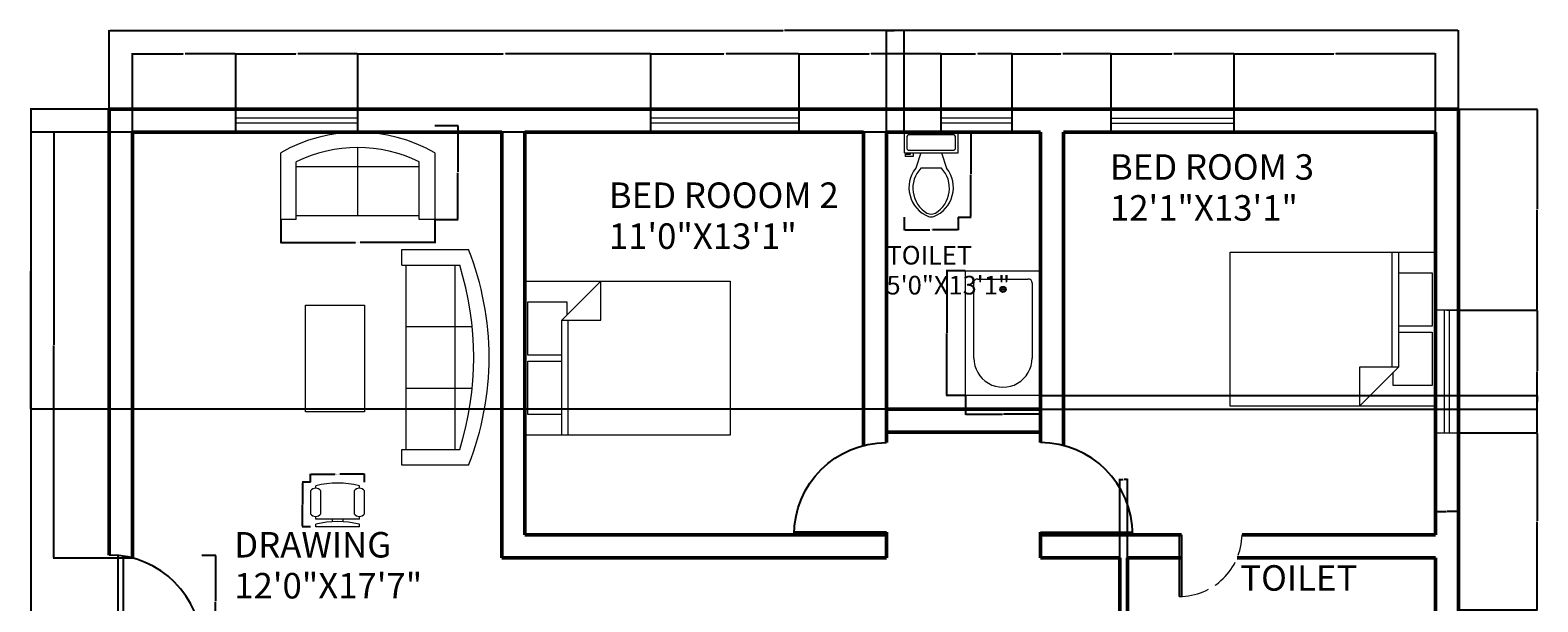
# Model space of a CAD drawing. Units: inches. Extents: x 614 to 1202, y 131 to 752.
# Tile 5 of 5: x 614 to 1202, y 529 to 752. Entities that reach past the tile are written whole.
import ezdxf

# ---------------------------------------------------------------- set-up
doc = ezdxf.new("R2010")
doc.units = ezdxf.units.IN
doc.header["$MEASUREMENT"] = 0
doc.linetypes.add('ACAD_ISO02W100', pattern=[15, 12, -3])
for name, color, linetype, lineweight in [('A-ANNO-DIMS', 2, 'Continuous', 18), ('A-AREA-IDEN', 7, 'Continuous', 18), ('A-DOOR', 3, 'Continuous', 25), ('A-DOOR-SWNG', 3, 'ACAD_ISO02W100', 13), ('A-FLOR-FIXT', 9, 'Continuous', 18), ('A-FURN', 8, 'Continuous', 18), ('A-GLAZ', 4, 'Continuous', 18), ('A-WALL', 7, 'Continuous', 50)]:
    doc.layers.add(name, color=color, linetype=linetype, lineweight=lineweight)
doc.styles.get("Standard").update_dxf_attribs({"font": 'arial.ttf'})
doc.dimstyles.get("Standard").update_dxf_attribs({"dimtxt": 0.18, "dimasz": 0.18, "dimexe": 0.18, "dimexo": 0.0625, "dimgap": 0.09, "dimtad": 0, "dimtih": 1, "dimtoh": 1, "dimdec": 0, "dimzin": 0, "dimdsep": 46, "dimlunit": 3, "dimtxsty": 'Standard', "dimcen": 0.09, "dimadec": 0, "dimazin": 0, "dimtfac": 1, "dimtdec": 0, "dimtofl": 0, "dimtmove": 0, "dimatfit": 3, "dimfxl": 1, "dimtolj": 1, "dimtzin": 0, "dimarcsym": 0})

# ---------------------------------------------------------------- blocks, each defined once
blk = doc.blocks.new('Sofa - Roundback Loveseat 5 ft.')
for p, q in [((-24, -33.99998), (-24, -11.46958)), ((0, -32.44198), (0, -5.99998)), ((24.00004, -33.99998), (24.00004, -11.46958)), ((-23.9998, -13.38178), (23.99986, -13.38178)), ((-24, -32.44198), (24.00004, -32.44198))]:
    blk.add_line(p, q)
for points in [[(-24, -33.99998), (-30, -33.99998), (-30, -7.99998)], [(30.00004, -7.99998), (30.00004, -33.99998), (24.00004, -33.99998)]]:
    blk.add_lwpolyline(points)
for centre, radius, start, end in [((0, -60.24998), 60.24998, 60.13715, 119.8628), ((0, -61.38438), 55.38444, 64.32083, 115.6792)]:
    blk.add_arc(centre, radius, start, end)
blk = doc.blocks.new('Sofa - Roundback 7 ft.')
for p, q in [((-36.000027, -34), (-36.000027, -11.4696)), ((-12.00002, -32.4421), (-12.00003, -6.5971)), ((11.99997, -32.4421), (11.99998, -6.5971)), ((35.99998, -34), (35.99998, -11.4696)), ((-35.999844, -13.3819), (35.9998, -13.3819)), ((-36.000027, -32.4421), (35.99998, -32.4421))]:
    blk.add_line(p, q)
for points in [[(-36.000027, -34), (-42.000027, -34), (-42.000027, -8)], [(41.99998, -8), (41.99998, -34), (35.99998, -34)]]:
    blk.add_lwpolyline(points)
for centre, radius, start, end in [((0, -114.25), 114.25, 68.43141, 111.5686), ((-0.00001, -127.1968), 121.1968, 72.72033, 107.2797)]:
    blk.add_arc(centre, radius, start, end)
blk = doc.blocks.new('Chair - Desk')
for p, q in [((-8.5, 0), (-8.5, -1)), ((-8.5, 0), (8.5, 0)), ((8.5, 0), (8.5, -1)), ((-10.5, -5), (-10.5, -14)), ((-8.5, -3), (-8.5, -4)), ((-8.5, -3), (8.5, -3)), ((-6.5, -14), (-6.5, -5)), ((-2, -3), (-2, -1.9355)), ((2, -1.9576), (2, -3)), ((6.5, -5), (6.5, -14)), ((8.5, -3), (8.5, -4)), ((10.5, -14), (10.5, -5)), ((-8.5, -15), (-8.5, -16)), ((8.5, -15), (8.5, -16))]:
    blk.add_line(p, q)
for centre, radius, start, end in [((-8.5, -6.5), 2.5, 36.8699, 143.1301), ((0, 34.625), 36.625, 256.5803, 283.4197), ((8.5, -6.5), 2.5, 36.8699, 143.1301), ((-8.5, -12.5), 2.5, 216.8699, 323.1301), ((0, 19.625), 36.625, 256.5803, 283.4197), ((8.5, -12.5), 2.5, 216.8699, 323.1301)]:
    blk.add_arc(centre, radius, start, end)
blk = doc.blocks.new('Bed - Queen')
for p, q in [((0, -80.00003), (0, 0)), ((0, 0), (59.99999, 0)), ((59.99999, 0), (59.99999, -80.00003)), ((7.99999, -1.2), (28.79998, -1.2)), ((7.99999, -14.4), (7.99999, -1.2)), ((28.79998, -1.2), (28.79998, -14.4)), ((31.19999, -1.2), (51.99999, -1.2)), ((31.19999, -14.4), (31.19999, -1.2)), ((51.99999, -1.2), (51.99999, -16.4)), ((0, -14.4), (44.8, -14.4)), ((44.8, -16.8), (0, -16.8)), ((59.99999, -29.6), (44.8, -14.4)), ((44.8, -14.4), (44.8, -29.6)), ((51.99999, -16.4), (46.79936, -16.4)), ((44.8, -29.6), (59.99999, -29.6)), ((59.99999, -80.00003), (0, -80.00003))]:
    blk.add_line(p, q)
blk = doc.blocks.new('Toilet - top')
for p, q in [((9.5, -6), (9.5, -2)), ((-10, -8.5), (-8, -8.5)), ((-10, -9.5), (-10, -8.5)), ((-7, -9.5), (-10, -9.5)), ((-8, -8.5), (-8, -8)), ((-7, -8), (-7, -9.5)), ((-4, -8), (-6, -14)), ((4, -8), (6, -14)), ((4, -14), (-4, -14))]:
    blk.add_line(p, q)
blk.add_lwpolyline([(10.5, -8), (10.5, 0), (-10.5, 0), (-10.5, -8)], close=True)
for points in [[(-9.5, -2), (-9.5, -6)], [(8.5, -1), (-8.5, -1)], [(-8.5, -7), (8.5, -7)]]:
    blk.add_lwpolyline(points)
for centre, radius, start, end in [((-8.62, -1.88), 0.884, 81.8699, 188.1301), ((8.62, -1.88), 0.884, 351.8699, 98.1301), ((-8.62, -6.12), 0.884, 171.8699, 278.1301), ((8.62, -6.12), 0.884, 261.8699, 8.1301), ((3.52, -21.58), 12.17, 141.46911, 247.97143), ((4.2, -21.82), 11.33, 136.36773, 238.94682), ((-3.52, -21.58), 12.17, 292.02843, 38.53071), ((-4.2, -21.82), 11.33, 301.05301, 43.63209), ((0, -27.88), 4, 245.73182, 294.26817), ((0, -29), 4, 254.86053, 285.13947)]:
    blk.add_arc(centre, radius, start, end)
blk = doc.blocks.new('Bath Tub - 26 x 60 in.')
for p, q in [((8, -18), (10, -18)), ((9, -17), (9, -19))]:
    blk.add_line(p, q)
blk.add_lwpolyline([(0, -36), (0, 0), (60, 0), (60, -36)], close=True)
for points in [[(4, -30), (4, -6)], [(6, -4), (42, -4)], [(42, -32), (6, -32)]]:
    blk.add_lwpolyline(points)
for radius in [1.5, 1]:
    blk.add_circle((9, -18), radius)
for centre, radius, start, end in [((5.75, -5.75), 1.77, 81.8699, 188.1301), ((42, -18), 14, 270, 90), ((5.75, -30.25), 1.77, 171.8699, 278.1301)]:
    blk.add_arc(centre, radius, start, end)
blk = doc.blocks.new('DOOR-SINGLE-36IN')
for p, q in [((0, 1), (36, 1)), ((0, 0), (36, 0))]:
    blk.add_line(p, q)
blk.add_arc((0, 0), 36, 0, 90)
blk = doc.blocks.new('*D11')
at = {"layer": 'A-ANNO-DIMS', "color": 0, "lineweight": -2, "transparency": 16777216}
for p, q in [((723.49, 575.83), (723.49, 579.1)), ((723.67, 578.92), (733.04, 578.92)), ((744.31, 578.92), (734.94, 578.92)), ((744.49, 575.83), (744.49, 579.1))]:
    blk.add_line(p, q, dxfattribs=at)
at = {"layer": 'A-ANNO-DIMS', "color": 0, "transparency": 16777216}
for points in [[(723.67, 578.95), (723.67, 578.89), (723.49, 578.92)], [(744.31, 578.95), (744.31, 578.89), (744.49, 578.92)]]:
    blk.add_solid(points, dxfattribs=at)
at = {"layer": 'Defpoints', "color": 0, "transparency": 16777216}
for p in [(723.49, 578.92), (723.49, 575.77), (744.49, 575.77)]:
    blk.add_point(p, dxfattribs=at)
at = {"layer": 'A-ANNO-DIMS', "color": 0, "transparency": 16777216, "insert": (733.99, 578.92), "char_height": 0.18, "attachment_point": 5}
blk.add_mtext('\\A1;CHAIR 21 TYP.', dxfattribs=at)
blk = doc.blocks.new('*D12')
at = {"layer": 'A-ANNO-DIMS', "color": 0, "lineweight": -2, "transparency": 16777216}
for p, q in [((723.43, 575.77), (720.16, 575.77)), ((720.34, 575.59), (720.34, 567.28)), ((720.34, 558.61), (720.34, 566.92)), ((723.43, 558.43), (720.16, 558.43))]:
    blk.add_line(p, q, dxfattribs=at)
at = {"layer": 'A-ANNO-DIMS', "color": 0, "transparency": 16777216}
for points in [[(720.31, 575.59), (720.37, 575.59), (720.34, 575.77)], [(720.31, 558.61), (720.37, 558.61), (720.34, 558.43)]]:
    blk.add_solid(points, dxfattribs=at)
at = {"layer": 'Defpoints', "color": 0, "transparency": 16777216}
for p in [(723.49, 575.77), (720.34, 558.43), (723.49, 558.43)]:
    blk.add_point(p, dxfattribs=at)
at = {"layer": 'A-ANNO-DIMS', "color": 0, "transparency": 16777216, "insert": (720.34, 567.1), "char_height": 0.18, "attachment_point": 5}
blk.add_mtext('\\A1;17 TYP.', dxfattribs=at)
blk = doc.blocks.new('*D15')
at = {"layer": 'A-ANNO-DIMS', "color": 0, "lineweight": -2, "transparency": 16777216}
for p, q in [((681.06, 547.36), (686.57, 547.36)), ((686.39, 547.18), (686.39, 529.54)), ((686.39, 511.54), (686.39, 529.18)), ((681.06, 511.36), (686.57, 511.36))]:
    blk.add_line(p, q, dxfattribs=at)
at = {"layer": 'A-ANNO-DIMS', "color": 0, "transparency": 16777216}
for points in [[(686.36, 547.18), (686.42, 547.18), (686.39, 547.36)], [(686.36, 511.54), (686.42, 511.54), (686.39, 511.36)]]:
    blk.add_solid(points, dxfattribs=at)
at = {"layer": 'Defpoints', "color": 0, "transparency": 16777216}
for p in [(680.99, 547.36), (686.39, 547.36), (680.99, 511.36)]:
    blk.add_point(p, dxfattribs=at)
at = {"layer": 'A-ANNO-DIMS', "color": 0, "transparency": 16777216, "insert": (686.39, 529.36), "char_height": 0.18, "attachment_point": 5}
blk.add_mtext('\\A1;DOOR 36 TYP.', dxfattribs=at)
blk = doc.blocks.new('*D19')
at = {"layer": 'A-ANNO-DIMS', "color": 0, "lineweight": -2, "transparency": 16777216}
for p, q in [((978.73, 658.26), (971.32, 658.26)), ((971.5, 658.08), (971.5, 634.11)), ((971.5, 609.78), (971.5, 633.75)), ((978.73, 609.6), (971.32, 609.6))]:
    blk.add_line(p, q, dxfattribs=at)
at = {"layer": 'A-ANNO-DIMS', "color": 0, "transparency": 16777216}
for points in [[(971.47, 658.08), (971.53, 658.08), (971.5, 658.26)], [(971.47, 609.78), (971.53, 609.78), (971.5, 609.6)]]:
    blk.add_solid(points, dxfattribs=at)
at = {"layer": 'Defpoints', "color": 0, "transparency": 16777216}
for p in [(978.8, 658.26), (971.5, 609.6), (978.8, 609.6)]:
    blk.add_point(p, dxfattribs=at)
at = {"layer": 'A-ANNO-DIMS', "color": 0, "transparency": 16777216, "insert": (971.5, 633.93), "char_height": 0.18, "attachment_point": 5}
blk.add_mtext('\\A1;TUB 49', dxfattribs=at)
blk = doc.blocks.new('*D20')
at = {"layer": 'A-ANNO-DIMS', "color": 0, "lineweight": -2, "transparency": 16777216}
for p, q in [((978.8, 609.54), (978.8, 602.12)), ((1007.99, 609.54), (1007.99, 602.12)), ((978.98, 602.3), (993.17, 602.3)), ((1007.81, 602.3), (993.62, 602.3))]:
    blk.add_line(p, q, dxfattribs=at)
at = {"layer": 'A-ANNO-DIMS', "color": 0, "transparency": 16777216}
for points in [[(978.98, 602.33), (978.98, 602.27), (978.8, 602.3)], [(1007.81, 602.33), (1007.81, 602.27), (1007.99, 602.3)]]:
    blk.add_solid(points, dxfattribs=at)
at = {"layer": 'Defpoints', "color": 0, "transparency": 16777216}
for p in [(978.8, 609.6), (1007.99, 609.6), (1007.99, 602.3)]:
    blk.add_point(p, dxfattribs=at)
at = {"layer": 'A-ANNO-DIMS', "color": 0, "transparency": 16777216, "insert": (993.4, 602.3), "char_height": 0.18, "attachment_point": 5}
blk.add_mtext('\\A1;29', dxfattribs=at)
blk = doc.blocks.new('*D21')
at = {"layer": 'A-ANNO-DIMS', "color": 0, "lineweight": -2, "transparency": 16777216}
for p, q in [((975.98, 712.26), (981.06, 712.26)), ((980.88, 712.08), (980.88, 695.92)), ((980.88, 679.4), (980.88, 695.56)), ((975.98, 679.22), (981.06, 679.22))]:
    blk.add_line(p, q, dxfattribs=at)
at = {"layer": 'A-ANNO-DIMS', "color": 0, "transparency": 16777216}
for points in [[(980.85, 712.08), (980.91, 712.08), (980.88, 712.26)], [(980.85, 679.4), (980.91, 679.4), (980.88, 679.22)]]:
    blk.add_solid(points, dxfattribs=at)
at = {"layer": 'Defpoints', "color": 0, "transparency": 16777216}
for p in [(975.92, 712.26), (980.88, 712.26), (975.92, 679.22)]:
    blk.add_point(p, dxfattribs=at)
at = {"layer": 'A-ANNO-DIMS', "color": 0, "transparency": 16777216, "insert": (980.88, 695.74), "char_height": 0.18, "attachment_point": 5}
blk.add_mtext('\\A1;WC 33 TYP.', dxfattribs=at)
blk = doc.blocks.new('*D22')
at = {"layer": 'A-ANNO-DIMS', "color": 0, "lineweight": -2, "transparency": 16777216}
for p, q in [((954.92, 679.15), (954.92, 674.08)), ((975.92, 679.15), (975.92, 674.08)), ((955.1, 674.26), (964.89, 674.26)), ((975.74, 674.26), (965.95, 674.26))]:
    blk.add_line(p, q, dxfattribs=at)
at = {"layer": 'A-ANNO-DIMS', "color": 0, "transparency": 16777216}
for points in [[(955.1, 674.29), (955.1, 674.23), (954.92, 674.26)], [(975.74, 674.29), (975.74, 674.23), (975.92, 674.26)]]:
    blk.add_solid(points, dxfattribs=at)
at = {"layer": 'Defpoints', "color": 0, "transparency": 16777216}
for p in [(954.92, 679.22), (975.92, 679.22), (975.92, 674.26)]:
    blk.add_point(p, dxfattribs=at)
at = {"layer": 'A-ANNO-DIMS', "color": 0, "transparency": 16777216, "insert": (965.42, 674.26), "char_height": 0.18, "attachment_point": 5}
blk.add_mtext('\\A1;21 TYP.', dxfattribs=at)
blk = doc.blocks.new('*D31')
at = {"layer": 'A-ANNO-DIMS', "color": 0, "lineweight": -2, "transparency": 16777216}
for p, q in [((711.85, 678.2), (711.85, 669.08)), ((771.85, 678.2), (771.85, 669.08)), ((712.03, 669.26), (740.94, 669.26)), ((771.67, 669.26), (742.76, 669.26))]:
    blk.add_line(p, q, dxfattribs=at)
at = {"layer": 'A-ANNO-DIMS', "color": 0, "transparency": 16777216}
for points in [[(712.03, 669.29), (712.03, 669.23), (711.85, 669.26)], [(771.67, 669.29), (771.67, 669.23), (771.85, 669.26)]]:
    blk.add_solid(points, dxfattribs=at)
at = {"layer": 'Defpoints', "color": 0, "transparency": 16777216}
for p in [(711.85, 678.26), (771.85, 678.26), (771.85, 669.26)]:
    blk.add_point(p, dxfattribs=at)
at = {"layer": 'A-ANNO-DIMS', "color": 0, "transparency": 16777216, "insert": (741.85, 669.26), "char_height": 0.18, "attachment_point": 5}
blk.add_mtext('\\A1;LOVESEAT 60', dxfattribs=at)
blk = doc.blocks.new('*D32')
at = {"layer": 'A-ANNO-DIMS', "color": 0, "lineweight": -2, "transparency": 16777216}
for p, q in [((771.91, 714.93), (781.03, 714.93)), ((780.85, 714.75), (780.85, 696.78)), ((780.85, 678.44), (780.85, 696.41)), ((771.91, 678.26), (781.03, 678.26))]:
    blk.add_line(p, q, dxfattribs=at)
at = {"layer": 'A-ANNO-DIMS', "color": 0, "transparency": 16777216}
for points in [[(780.82, 714.75), (780.88, 714.75), (780.85, 714.93)], [(780.82, 678.44), (780.88, 678.44), (780.85, 678.26)]]:
    blk.add_solid(points, dxfattribs=at)
at = {"layer": 'Defpoints', "color": 0, "transparency": 16777216}
for p in [(771.85, 714.93), (780.85, 714.93), (771.85, 678.26)]:
    blk.add_point(p, dxfattribs=at)
at = {"layer": 'A-ANNO-DIMS', "color": 0, "transparency": 16777216, "insert": (780.85, 696.6), "char_height": 0.18, "attachment_point": 5}
blk.add_mtext('\\A1;37', dxfattribs=at)
blk = doc.blocks.new('*D35')
at = {"layer": 'A-ANNO-DIMS', "color": 0, "lineweight": -2, "transparency": 16777216}
for p, q in [((644.99, 721.33), (644.99, 752.09)), ((645.17, 751.91), (907.7, 751.91)), ((1170.81, 751.91), (908.28, 751.91)), ((1170.99, 721.33), (1170.99, 752.09))]:
    blk.add_line(p, q, dxfattribs=at)
at = {"layer": 'A-ANNO-DIMS', "color": 0, "transparency": 16777216}
for points in [[(645.17, 751.94), (645.17, 751.88), (644.99, 751.91)], [(1170.81, 751.94), (1170.81, 751.88), (1170.99, 751.91)]]:
    blk.add_solid(points, dxfattribs=at)
at = {"layer": 'Defpoints', "color": 0, "transparency": 16777216}
for p in [(1170.99, 751.91), (644.99, 721.26), (1170.99, 721.26)]:
    blk.add_point(p, dxfattribs=at)
at = {"layer": 'A-ANNO-DIMS', "color": 0, "transparency": 16777216, "insert": (907.99, 751.91), "char_height": 0.18, "attachment_point": 5}
blk.add_mtext('\\A1;526', dxfattribs=at)
blk = doc.blocks.new('*D36')
at = {"layer": 'A-ANNO-DIMS', "color": 0, "lineweight": -2, "transparency": 16777216}
for p, q in [((644.93, 721.26), (614.16, 721.26)), ((614.34, 721.08), (614.34, 441.95)), ((614.34, 162.44), (614.34, 441.58)), ((857.93, 162.26), (614.16, 162.26))]:
    blk.add_line(p, q, dxfattribs=at)
at = {"layer": 'A-ANNO-DIMS', "color": 0, "transparency": 16777216}
for points in [[(614.31, 721.08), (614.37, 721.08), (614.34, 721.26)], [(614.31, 162.44), (614.37, 162.44), (614.34, 162.26)]]:
    blk.add_solid(points, dxfattribs=at)
at = {"layer": 'Defpoints', "color": 0, "transparency": 16777216}
for p in [(614.34, 721.26), (644.99, 721.26), (857.99, 162.26)]:
    blk.add_point(p, dxfattribs=at)
at = {"layer": 'A-ANNO-DIMS', "color": 0, "transparency": 16777216, "insert": (614.34, 441.76), "char_height": 0.18, "attachment_point": 5}
blk.add_mtext('\\A1;559', dxfattribs=at)
blk = doc.blocks.new('*D37')
at = {"layer": 'A-ANNO-DIMS', "color": 0, "lineweight": -2, "transparency": 16777216}
for p, q in [((653.99, 712.33), (653.99, 743.09)), ((654.17, 742.91), (673.77, 742.91)), ((694.12, 742.91), (674.53, 742.91)), ((694.3, 712.33), (694.3, 743.09))]:
    blk.add_line(p, q, dxfattribs=at)
at = {"layer": 'A-ANNO-DIMS', "color": 0, "transparency": 16777216}
for points in [[(654.17, 742.94), (654.17, 742.88), (653.99, 742.91)], [(694.12, 742.94), (694.12, 742.88), (694.3, 742.91)]]:
    blk.add_solid(points, dxfattribs=at)
at = {"layer": 'Defpoints', "color": 0, "transparency": 16777216}
for p in [(694.3, 742.91), (653.99, 712.26), (694.3, 712.26)]:
    blk.add_point(p, dxfattribs=at)
at = {"layer": 'A-ANNO-DIMS', "color": 0, "transparency": 16777216, "insert": (674.15, 742.91), "char_height": 0.18, "attachment_point": 5}
blk.add_mtext('\\A1;40.31', dxfattribs=at)
blk = doc.blocks.new('*D38')
at = {"layer": 'A-ANNO-DIMS', "color": 0, "lineweight": -2, "transparency": 16777216}
for p, q in [((694.3, 712.33), (694.3, 743.09)), ((694.48, 742.91), (717.68, 742.91)), ((741.67, 742.91), (718.47, 742.91)), ((741.85, 712.33), (741.85, 743.09))]:
    blk.add_line(p, q, dxfattribs=at)
at = {"layer": 'A-ANNO-DIMS', "color": 0, "transparency": 16777216}
for points in [[(694.48, 742.94), (694.48, 742.88), (694.3, 742.91)], [(741.67, 742.94), (741.67, 742.88), (741.85, 742.91)]]:
    blk.add_solid(points, dxfattribs=at)
at = {"layer": 'Defpoints', "color": 0, "transparency": 16777216}
for p in [(741.85, 742.91), (694.3, 712.26), (741.85, 712.26)]:
    blk.add_point(p, dxfattribs=at)
at = {"layer": 'A-ANNO-DIMS', "color": 0, "transparency": 16777216, "insert": (718.08, 742.91), "char_height": 0.18, "attachment_point": 5}
blk.add_mtext('\\A1;47.55', dxfattribs=at)
blk = doc.blocks.new('*D39')
at = {"layer": 'A-ANNO-DIMS', "color": 0, "lineweight": -2, "transparency": 16777216}
for p, q in [((741.85, 712.33), (741.85, 743.09)), ((742.03, 742.91), (798.56, 742.91)), ((856.01, 742.91), (799.47, 742.91)), ((856.19, 712.33), (856.19, 743.09))]:
    blk.add_line(p, q, dxfattribs=at)
at = {"layer": 'A-ANNO-DIMS', "color": 0, "transparency": 16777216}
for points in [[(742.03, 742.94), (742.03, 742.88), (741.85, 742.91)], [(856.01, 742.94), (856.01, 742.88), (856.19, 742.91)]]:
    blk.add_solid(points, dxfattribs=at)
at = {"layer": 'Defpoints', "color": 0, "transparency": 16777216}
for p in [(856.19, 742.91), (741.85, 712.26), (856.19, 712.26)]:
    blk.add_point(p, dxfattribs=at)
at = {"layer": 'A-ANNO-DIMS', "color": 0, "transparency": 16777216, "insert": (799.02, 742.91), "char_height": 0.18, "attachment_point": 5}
blk.add_mtext('\\A1;114.34', dxfattribs=at)
blk = doc.blocks.new('*D40')
at = {"layer": 'A-ANNO-DIMS', "color": 0, "lineweight": -2, "transparency": 16777216}
for p, q in [((856.19, 712.33), (856.19, 743.09)), ((856.37, 742.91), (884.65, 742.91)), ((913.72, 742.91), (885.44, 742.91)), ((913.9, 712.33), (913.9, 743.09))]:
    blk.add_line(p, q, dxfattribs=at)
at = {"layer": 'A-ANNO-DIMS', "color": 0, "transparency": 16777216}
for points in [[(856.37, 742.94), (856.37, 742.88), (856.19, 742.91)], [(913.72, 742.94), (913.72, 742.88), (913.9, 742.91)]]:
    blk.add_solid(points, dxfattribs=at)
at = {"layer": 'Defpoints', "color": 0, "transparency": 16777216}
for p in [(913.9, 742.91), (856.19, 712.26), (913.9, 712.26)]:
    blk.add_point(p, dxfattribs=at)
at = {"layer": 'A-ANNO-DIMS', "color": 0, "transparency": 16777216, "insert": (885.04, 742.91), "char_height": 0.18, "attachment_point": 5}
blk.add_mtext('\\A1;57.72', dxfattribs=at)
blk = doc.blocks.new('*D41')
at = {"layer": 'A-ANNO-DIMS', "color": 0, "lineweight": -2, "transparency": 16777216}
for p, q in [((913.9, 712.33), (913.9, 743.09)), ((914.08, 742.91), (941.25, 742.91)), ((969.2, 742.91), (942.04, 742.91)), ((969.38, 712.33), (969.38, 743.09))]:
    blk.add_line(p, q, dxfattribs=at)
at = {"layer": 'A-ANNO-DIMS', "color": 0, "transparency": 16777216}
for points in [[(914.08, 742.94), (914.08, 742.88), (913.9, 742.91)], [(969.2, 742.94), (969.2, 742.88), (969.38, 742.91)]]:
    blk.add_solid(points, dxfattribs=at)
at = {"layer": 'Defpoints', "color": 0, "transparency": 16777216}
for p in [(969.38, 742.91), (913.9, 712.26), (969.38, 712.26)]:
    blk.add_point(p, dxfattribs=at)
at = {"layer": 'A-ANNO-DIMS', "color": 0, "transparency": 16777216, "insert": (941.64, 742.91), "char_height": 0.18, "attachment_point": 5}
blk.add_mtext('\\A1;55.48', dxfattribs=at)
blk = doc.blocks.new('*D42')
at = {"layer": 'A-ANNO-DIMS', "color": 0, "lineweight": -2, "transparency": 16777216}
for p, q in [((969.38, 712.33), (969.38, 743.09)), ((969.56, 742.91), (982.74, 742.91)), ((996.86, 742.91), (983.67, 742.91)), ((997.04, 712.33), (997.04, 743.09))]:
    blk.add_line(p, q, dxfattribs=at)
at = {"layer": 'A-ANNO-DIMS', "color": 0, "transparency": 16777216}
for points in [[(969.56, 742.94), (969.56, 742.88), (969.38, 742.91)], [(996.86, 742.94), (996.86, 742.88), (997.04, 742.91)]]:
    blk.add_solid(points, dxfattribs=at)
at = {"layer": 'Defpoints', "color": 0, "transparency": 16777216}
for p in [(997.04, 742.91), (969.38, 712.26), (997.04, 712.26)]:
    blk.add_point(p, dxfattribs=at)
at = {"layer": 'A-ANNO-DIMS', "color": 0, "transparency": 16777216, "insert": (983.21, 742.91), "char_height": 0.18, "attachment_point": 5}
blk.add_mtext('\\A1;27.657', dxfattribs=at)
blk = doc.blocks.new('*D43')
at = {"layer": 'A-ANNO-DIMS', "color": 0, "lineweight": -2, "transparency": 16777216}
for p, q in [((997.04, 712.33), (997.04, 743.09)), ((997.22, 742.91), (1015.94, 742.91)), ((1035.45, 742.91), (1016.73, 742.91)), ((1035.63, 712.33), (1035.63, 743.09))]:
    blk.add_line(p, q, dxfattribs=at)
at = {"layer": 'A-ANNO-DIMS', "color": 0, "transparency": 16777216}
for points in [[(997.22, 742.94), (997.22, 742.88), (997.04, 742.91)], [(1035.45, 742.94), (1035.45, 742.88), (1035.63, 742.91)]]:
    blk.add_solid(points, dxfattribs=at)
at = {"layer": 'Defpoints', "color": 0, "transparency": 16777216}
for p in [(1035.63, 742.91), (997.04, 712.26), (1035.63, 712.26)]:
    blk.add_point(p, dxfattribs=at)
at = {"layer": 'A-ANNO-DIMS', "color": 0, "transparency": 16777216, "insert": (1016.33, 742.91), "char_height": 0.18, "attachment_point": 5}
blk.add_mtext('\\A1;38.59', dxfattribs=at)
blk = doc.blocks.new('*D44')
at = {"layer": 'A-ANNO-DIMS', "color": 0, "lineweight": -2, "transparency": 16777216}
for p, q in [((1035.63, 712.33), (1035.63, 743.09)), ((1035.81, 742.91), (1059.22, 742.91)), ((1083.43, 742.91), (1060.02, 742.91)), ((1083.61, 712.33), (1083.61, 743.09))]:
    blk.add_line(p, q, dxfattribs=at)
at = {"layer": 'A-ANNO-DIMS', "color": 0, "transparency": 16777216}
for points in [[(1035.81, 742.94), (1035.81, 742.88), (1035.63, 742.91)], [(1083.43, 742.94), (1083.43, 742.88), (1083.61, 742.91)]]:
    blk.add_solid(points, dxfattribs=at)
at = {"layer": 'Defpoints', "color": 0, "transparency": 16777216}
for p in [(1083.61, 742.91), (1035.63, 712.26), (1083.61, 712.26)]:
    blk.add_point(p, dxfattribs=at)
at = {"layer": 'A-ANNO-DIMS', "color": 0, "transparency": 16777216, "insert": (1059.62, 742.91), "char_height": 0.18, "attachment_point": 5}
blk.add_mtext('\\A1;47.99', dxfattribs=at)
blk = doc.blocks.new('*D45')
at = {"layer": 'A-ANNO-DIMS', "color": 0, "lineweight": -2, "transparency": 16777216}
for p, q in [((1083.61, 712.33), (1083.61, 743.09)), ((1083.79, 742.91), (1122.41, 742.91)), ((1161.81, 742.91), (1123.2, 742.91)), ((1161.99, 712.33), (1161.99, 743.09))]:
    blk.add_line(p, q, dxfattribs=at)
at = {"layer": 'A-ANNO-DIMS', "color": 0, "transparency": 16777216}
for points in [[(1083.79, 742.94), (1083.79, 742.88), (1083.61, 742.91)], [(1161.81, 742.94), (1161.81, 742.88), (1161.99, 742.91)]]:
    blk.add_solid(points, dxfattribs=at)
at = {"layer": 'Defpoints', "color": 0, "transparency": 16777216}
for p in [(1161.99, 742.91), (1083.61, 712.26), (1161.99, 712.26)]:
    blk.add_point(p, dxfattribs=at)
at = {"layer": 'A-ANNO-DIMS', "color": 0, "transparency": 16777216, "insert": (1122.8, 742.91), "char_height": 0.18, "attachment_point": 5}
blk.add_mtext('\\A1;78.38', dxfattribs=at)
blk = doc.blocks.new('*D46')
at = {"layer": 'A-ANNO-DIMS', "color": 0, "lineweight": -2, "transparency": 16777216}
for p, q in [((653.93, 712.26), (623.16, 712.26)), ((623.34, 712.08), (623.34, 629.42)), ((623.34, 546.4), (623.34, 629.06)), ((653.93, 546.22), (623.16, 546.22))]:
    blk.add_line(p, q, dxfattribs=at)
at = {"layer": 'A-ANNO-DIMS', "color": 0, "transparency": 16777216}
for points in [[(623.31, 712.08), (623.37, 712.08), (623.34, 712.26)], [(623.31, 546.4), (623.37, 546.4), (623.34, 546.22)]]:
    blk.add_solid(points, dxfattribs=at)
at = {"layer": 'Defpoints', "color": 0, "transparency": 16777216}
for p in [(623.34, 712.26), (653.99, 712.26), (653.99, 546.22)]:
    blk.add_point(p, dxfattribs=at)
at = {"layer": 'A-ANNO-DIMS', "color": 0, "transparency": 16777216, "insert": (623.34, 629.24), "char_height": 0.18, "attachment_point": 5}
blk.add_mtext('\\A1;166.05', dxfattribs=at)
blk = doc.blocks.new('*D52')
at = {"layer": 'A-ANNO-DIMS', "color": 0, "lineweight": -2, "transparency": 16777216}
for p, q in [((1171.06, 721.26), (1201.82, 721.26)), ((1201.64, 721.08), (1201.64, 682.28)), ((1201.64, 643.12), (1201.64, 681.92)), ((1171.06, 642.94), (1201.82, 642.94))]:
    blk.add_line(p, q, dxfattribs=at)
at = {"layer": 'A-ANNO-DIMS', "color": 0, "transparency": 16777216}
for points in [[(1201.61, 721.08), (1201.67, 721.08), (1201.64, 721.26)], [(1201.61, 643.12), (1201.67, 643.12), (1201.64, 642.94)]]:
    blk.add_solid(points, dxfattribs=at)
at = {"layer": 'Defpoints', "color": 0, "transparency": 16777216}
for p in [(1170.99, 721.26), (1201.64, 721.26), (1170.99, 642.94)]:
    blk.add_point(p, dxfattribs=at)
at = {"layer": 'A-ANNO-DIMS', "color": 0, "transparency": 16777216, "insert": (1201.64, 682.1), "char_height": 0.18, "attachment_point": 5}
blk.add_mtext('\\A1;78.32', dxfattribs=at)
blk = doc.blocks.new('*D53')
at = {"layer": 'A-ANNO-DIMS', "color": 0, "lineweight": -2, "transparency": 16777216}
for p, q in [((1171.06, 642.94), (1201.82, 642.94)), ((1201.64, 642.76), (1201.64, 619.15)), ((1201.64, 595.18), (1201.64, 618.79)), ((1171.06, 595), (1201.82, 595))]:
    blk.add_line(p, q, dxfattribs=at)
at = {"layer": 'A-ANNO-DIMS', "color": 0, "transparency": 16777216}
for points in [[(1201.61, 642.76), (1201.67, 642.76), (1201.64, 642.94)], [(1201.61, 595.18), (1201.67, 595.18), (1201.64, 595)]]:
    blk.add_solid(points, dxfattribs=at)
at = {"layer": 'Defpoints', "color": 0, "transparency": 16777216}
for p in [(1170.99, 642.94), (1201.64, 642.94), (1170.99, 595)]:
    blk.add_point(p, dxfattribs=at)
at = {"layer": 'A-ANNO-DIMS', "color": 0, "transparency": 16777216, "insert": (1201.64, 618.97), "char_height": 0.18, "attachment_point": 5}
blk.add_mtext('\\A1;47.94', dxfattribs=at)
blk = doc.blocks.new('*D54')
at = {"layer": 'A-ANNO-DIMS', "color": 0, "lineweight": -2, "transparency": 16777216}
for p, q in [((1171.06, 595), (1201.82, 595)), ((1201.64, 594.82), (1201.64, 560.69)), ((1201.64, 526.2), (1201.64, 560.33)), ((1171.06, 526.02), (1201.82, 526.02))]:
    blk.add_line(p, q, dxfattribs=at)
at = {"layer": 'A-ANNO-DIMS', "color": 0, "transparency": 16777216}
for points in [[(1201.61, 594.82), (1201.67, 594.82), (1201.64, 595)], [(1201.61, 526.2), (1201.67, 526.2), (1201.64, 526.02)]]:
    blk.add_solid(points, dxfattribs=at)
at = {"layer": 'Defpoints', "color": 0, "transparency": 16777216}
for p in [(1170.99, 595), (1201.64, 595), (1170.99, 526.02)]:
    blk.add_point(p, dxfattribs=at)
at = {"layer": 'A-ANNO-DIMS', "color": 0, "transparency": 16777216, "insert": (1201.64, 560.51), "char_height": 0.18, "attachment_point": 5}
blk.add_mtext('\\A1;68.99', dxfattribs=at)
blk = doc.blocks.new('*D70')
at = {"layer": 'A-ANNO-DIMS', "color": 0, "lineweight": -2, "transparency": 16777216}
for p, q in [((1161.99, 594.94), (1161.99, 564.17)), ((1170.99, 594.94), (1170.99, 564.17)), ((1162.17, 564.35), (1166.34, 564.35)), ((1170.81, 564.35), (1166.64, 564.35))]:
    blk.add_line(p, q, dxfattribs=at)
at = {"layer": 'A-ANNO-DIMS', "color": 0, "transparency": 16777216}
for points in [[(1162.17, 564.38), (1162.17, 564.32), (1161.99, 564.35)], [(1170.81, 564.38), (1170.81, 564.32), (1170.99, 564.35)]]:
    blk.add_solid(points, dxfattribs=at)
at = {"layer": 'Defpoints', "color": 0, "transparency": 16777216}
for p in [(1161.99, 595), (1170.99, 595), (1161.99, 564.35)]:
    blk.add_point(p, dxfattribs=at)
at = {"layer": 'A-ANNO-DIMS', "color": 0, "transparency": 16777216, "insert": (1166.49, 564.35), "char_height": 0.18, "attachment_point": 5}
blk.add_mtext('\\A1;9', dxfattribs=at)
blk = doc.blocks.new('*D72')
at = {"layer": 'A-ANNO-DIMS', "color": 0, "lineweight": -2, "transparency": 16777216}
for p, q in [((1038.99, 546.33), (1038.99, 577.09)), ((1039.17, 576.91), (1040.34, 576.91)), ((1041.81, 576.91), (1040.64, 576.91)), ((1041.99, 546.33), (1041.99, 577.09))]:
    blk.add_line(p, q, dxfattribs=at)
at = {"layer": 'A-ANNO-DIMS', "color": 0, "transparency": 16777216}
for points in [[(1039.17, 576.94), (1039.17, 576.88), (1038.99, 576.91)], [(1041.81, 576.94), (1041.81, 576.88), (1041.99, 576.91)]]:
    blk.add_solid(points, dxfattribs=at)
at = {"layer": 'Defpoints', "color": 0, "transparency": 16777216}
for p in [(1041.99, 576.91), (1038.99, 546.26), (1041.99, 546.26)]:
    blk.add_point(p, dxfattribs=at)
at = {"layer": 'A-ANNO-DIMS', "color": 0, "transparency": 16777216, "insert": (1040.49, 576.91), "char_height": 0.18, "attachment_point": 5}
blk.add_mtext('\\A1;3', dxfattribs=at)
blk = doc.blocks.new('*D73')
at = {"layer": 'A-ANNO-DIMS', "color": 0, "lineweight": -2, "transparency": 16777216}
for p, q in [((947.93, 712.26), (614.16, 712.26)), ((614.34, 712.08), (614.34, 658.45)), ((614.34, 604.44), (614.34, 658.08)), ((947.93, 604.26), (614.16, 604.26))]:
    blk.add_line(p, q, dxfattribs=at)
at = {"layer": 'A-ANNO-DIMS', "color": 0, "transparency": 16777216}
for points in [[(614.31, 712.08), (614.37, 712.08), (614.34, 712.26)], [(614.31, 604.44), (614.37, 604.44), (614.34, 604.26)]]:
    blk.add_solid(points, dxfattribs=at)
at = {"layer": 'Defpoints', "color": 0, "transparency": 16777216}
for p in [(614.34, 712.26), (947.99, 712.26), (947.99, 604.26)]:
    blk.add_point(p, dxfattribs=at)
at = {"layer": 'A-ANNO-DIMS', "color": 0, "transparency": 16777216, "insert": (614.34, 658.26), "char_height": 0.18, "attachment_point": 5}
blk.add_mtext('\\A1;108', dxfattribs=at)
blk = doc.blocks.new('*D74')
at = {"layer": 'A-ANNO-DIMS', "color": 0, "lineweight": -2, "transparency": 16777216}
for p, q in [((947.99, 712.33), (947.99, 752.09)), ((948.17, 751.91), (951.06, 751.91)), ((954.74, 751.91), (951.85, 751.91)), ((954.92, 712.33), (954.92, 752.09))]:
    blk.add_line(p, q, dxfattribs=at)
at = {"layer": 'A-ANNO-DIMS', "color": 0, "transparency": 16777216}
for points in [[(948.17, 751.94), (948.17, 751.88), (947.99, 751.91)], [(954.74, 751.94), (954.74, 751.88), (954.92, 751.91)]]:
    blk.add_solid(points, dxfattribs=at)
at = {"layer": 'Defpoints', "color": 0, "transparency": 16777216}
for p in [(954.92, 751.91), (947.99, 712.26), (954.92, 712.26)]:
    blk.add_point(p, dxfattribs=at)
at = {"layer": 'A-ANNO-DIMS', "color": 0, "transparency": 16777216, "insert": (951.46, 751.91), "char_height": 0.18, "attachment_point": 5}
blk.add_mtext('\\A1;6.927', dxfattribs=at)
blk = doc.blocks.new('*D75')
at = {"layer": 'A-ANNO-DIMS', "color": 0, "lineweight": -2, "transparency": 16777216}
for p, q in [((1008.06, 609.6), (1201.82, 609.6)), ((1201.64, 609.42), (1201.64, 607.11)), ((1201.64, 604.44), (1201.64, 606.75)), ((1008.06, 604.26), (1201.82, 604.26))]:
    blk.add_line(p, q, dxfattribs=at)
at = {"layer": 'A-ANNO-DIMS', "color": 0, "transparency": 16777216}
for points in [[(1201.61, 609.42), (1201.67, 609.42), (1201.64, 609.6)], [(1201.61, 604.44), (1201.67, 604.44), (1201.64, 604.26)]]:
    blk.add_solid(points, dxfattribs=at)
at = {"layer": 'Defpoints', "color": 0, "transparency": 16777216}
for p in [(1007.99, 609.6), (1201.64, 609.6), (1007.99, 604.26)]:
    blk.add_point(p, dxfattribs=at)
at = {"layer": 'A-ANNO-DIMS', "color": 0, "transparency": 16777216, "insert": (1201.64, 606.93), "char_height": 0.18, "attachment_point": 5}
blk.add_mtext('\\A1;5.338', dxfattribs=at)

msp = doc.modelspace()

# ---------------------------------------------------------------- linework, layer by layer
at = {"layer": 'A-DOOR'}
for p, q in [((947.9938, 555.2636), (947.9938, 556.2636)), ((1062.0637, 555.2636), (1062.0637, 531.1925)), ((1062.0637, 555.2636), (1063.0637, 555.2636)), ((1063.0637, 555.2636), (1063.0637, 531.1925)), ((648.4938, 511.3589), (648.4938, 547.1883)), ((650.4938, 511.3589), (650.4938, 546.9362))]:
    msp.add_line(p, q, dxfattribs=at)
at = {"layer": 'A-DOOR-SWNG'}
msp.add_arc((1062.0637, 555.7692), 24.5767, 270, 358.8212034, dxfattribs=at)
at = {"layer": 'A-FURN'}
msp.add_lwpolyline([(721.4854, 644.8133), (744.5569, 644.8133), (744.5569, 603.2003), (721.4854, 603.2003)], close=True, dxfattribs=at)
at = {"layer": 'A-GLAZ'}
for p, q in [((694.303, 716.7636), (694.303, 721.2636)), ((694.303, 721.2636), (694.303, 712.2636)), ((741.8501, 717.7636), (694.303, 717.7636)), ((741.8501, 721.2636), (741.8501, 712.2636)), ((856.1868, 716.7636), (856.1868, 721.2636)), ((856.1868, 721.2636), (856.1868, 712.2636)), ((913.903, 717.7636), (856.1868, 717.7636)), ((913.903, 712.2636), (913.903, 721.2636)), ((969.3793, 716.7636), (969.3793, 721.2636)), ((969.3793, 721.2636), (969.3793, 712.2636)), ((997.0359, 717.7636), (969.3793, 717.7636)), ((997.0359, 712.2636), (997.0359, 721.2636)), ((1035.627, 721.2636), (1035.627, 712.2636)), ((1035.627, 717.7636), (1083.6132, 717.7636)), ((1083.6132, 716.7636), (1083.6132, 721.2636)), ((1083.6132, 721.2636), (1083.6132, 712.2636)), ((741.8501, 715.7636), (694.303, 715.7636)), ((913.903, 715.7636), (856.1868, 715.7636)), ((997.0359, 715.7636), (969.3793, 715.7636)), ((1035.627, 715.7636), (1083.6132, 715.7636)), ((1170.9938, 642.9424), (1161.9938, 642.9424)), ((1165.4938, 595.0017), (1165.4938, 642.9424)), ((1166.4938, 642.9424), (1170.9938, 642.9424)), ((1167.4938, 595.0017), (1167.4938, 642.9424)), ((1161.9938, 595.0017), (1170.9938, 595.0017))]:
    msp.add_line(p, q, dxfattribs=at)
at = {"layer": 'A-WALL'}
for p, q in [((644.9938, 721.2636), (644.9938, 547.3589)), ((644.9938, 721.2636), (1170.9938, 721.2636)), ((653.9938, 721.2636), (797.9938, 721.2636)), ((806.9938, 721.2636), (938.9938, 721.2636)), ((947.9938, 721.2636), (1007.9938, 721.2636)), ((1170.9938, 721.2636), (1170.9938, 222.2636)), ((653.9938, 712.2636), (797.9938, 712.2636)), ((653.9938, 712.2636), (653.9938, 546.2157)), ((797.9938, 712.2636), (797.9938, 546.2636)), ((806.9938, 712.2636), (806.9938, 555.2636)), ((806.9938, 712.2636), (938.9938, 712.2636)), ((938.9938, 712.2636), (938.9938, 590.1204)), ((947.9938, 712.2636), (947.9938, 591.2636)), ((947.9938, 712.2636), (1007.9938, 712.2636)), ((1007.9938, 712.2636), (1007.9938, 604.2636)), ((1016.9938, 712.2636), (1016.9938, 604.2636)), ((1016.9938, 712.2636), (1161.9938, 712.2636)), ((1161.9938, 712.2636), (1161.9938, 555.2636)), ((1170.9938, 712.2636), (1170.9938, 555.2636)), ((1007.9938, 604.2636), (947.9938, 604.2636)), ((1007.9938, 591.2636), (1007.9938, 604.2636)), ((1016.9938, 590.1204), (1016.9938, 604.2636)), ((1007.9938, 595.2636), (947.9938, 595.2636)), ((947.9938, 555.2636), (806.9938, 555.2636)), ((938.9938, 556.2636), (938.9938, 555.2636)), ((947.9938, 556.2636), (947.9938, 546.2636)), ((1007.9938, 546.2636), (1007.9938, 556.2636)), ((1063.0637, 555.2636), (1007.9938, 555.2636)), ((1016.9938, 555.2636), (1016.9938, 556.2636)), ((1161.9938, 555.2636), (1086.6352, 555.2636)), ((947.9938, 546.2636), (797.9938, 546.2636)), ((1038.9938, 546.2636), (1007.9938, 546.2636)), ((1038.9938, 486.2636), (1038.9938, 546.2636)), ((1041.9938, 486.2636), (1041.9938, 546.2636)), ((1063.0637, 546.2636), (1041.9938, 546.2636)), ((1161.9938, 546.2636), (1084.7277, 546.2636)), ((1161.9938, 546.2636), (1161.9938, 486.2636)), ((1170.9938, 546.2636), (1170.9938, 486.2636))]:
    msp.add_line(p, q, dxfattribs=at)

# ---------------------------------------------------------------- block references
at = {"layer": 'A-DOOR', "extrusion": (0, 0, -1), "zscale": -1}
msp.add_blockref('DOOR-SINGLE-36IN', (-947.9935, 555.2637), dxfattribs=at)
at = {"layer": 'A-DOOR'}
for p in [(1007.994, 555.2637), (644.994, 511.359)]:
    msp.add_blockref('DOOR-SINGLE-36IN', p, dxfattribs=at)
at = {"layer": 'A-FLOR-FIXT'}
msp.add_blockref('Toilet - top', (965.4207, 712.2636), dxfattribs=at)
at = {"layer": 'A-FLOR-FIXT', "xscale": 0.8110350040397625, "yscale": 0.8110350040397625, "zscale": 0.8110350040397625, "rotation": 270}
msp.add_blockref('Bath Tub - 26 x 60 in.', (1007.9938, 658.2636), dxfattribs=at)
at = {"layer": 'A-FURN'}
msp.add_blockref('Sofa - Roundback Loveseat 5 ft.', (741.8501, 712.2636), dxfattribs=at)
for name, p, rotation in [('Sofa - Roundback 7 ft.', (793.0823, 624.486), 270), ('Bed - Queen', (1161.9938, 665.4617), 270), ('Bed - Queen', (806.9938, 594.1968), 90), ('Chair - Desk', (733.9905, 558.4322), 180)]:
    msp.add_blockref(name, p, dxfattribs=dict(at, rotation=rotation))

# ---------------------------------------------------------------- texts
at = {"layer": 'A-AREA-IDEN'}
for s, height, p in [('BED ROOM 3', 9.93672, (1035.1195, 693.7635)), ('BED ROOOM 2', 9.93672, (839.7467, 682.7522)), ('12\'1"X13\'1"', 9.93672, (1035.1195, 677.801)), ('11\'0"X13\'1"', 9.93672, (839.7467, 666.7898)), ('TOILET ', 7.27583, (947.9938, 660.6856)), ('5\'0"X13\'1"', 7.27583, (947.9938, 648.9976)), ('DRAWING ', 9.93672, (693.7057, 546.421)), ('12\'0"X17\'7"', 9.93672, (693.7057, 530.4585)), ('TOILET ', 9.93672, (1085.9373, 533.4854))]:
    msp.add_text(s, height=height, dxfattribs=at).set_placement(p)

# ---------------------------------------------------------------- dimensions: what is measured, and where the dimension line sits
at = {"layer": 'A-ANNO-DIMS'}
for base, p1, p2, override, picture, middle in [((1170.9938, 751.9136), (644.9938, 721.2636), (1170.9938, 721.2636), {"dimdec": 0, "dimlfac": 1, "dimrnd": 0, "dimzin": 0, "dimdsep": 46, "dimlunit": 2}, '*D35', (907.9938, 751.9136)), ((954.9207, 751.9136), (947.9938, 712.2636), (954.9207, 712.2636), {"dimdec": 3, "dimlfac": 1, "dimrnd": 0, "dimzin": 0, "dimdsep": 46, "dimlunit": 2}, '*D74', (951.4572, 751.9136)), ((694.303, 742.9136), (653.9938, 712.2636), (694.303, 712.2636), {"dimdec": 2, "dimlfac": 1, "dimrnd": 0, "dimzin": 0, "dimdsep": 46, "dimlunit": 2}, '*D37', (674.1484, 742.9136)), ((741.8501, 742.9136), (694.303, 712.2636), (741.8501, 712.2636), {"dimdec": 2, "dimlfac": 1, "dimrnd": 0, "dimzin": 0, "dimdsep": 46, "dimlunit": 2}, '*D38', (718.0766, 742.9136)), ((856.1868, 742.9136), (741.8501, 712.2636), (856.1868, 712.2636), {"dimdec": 2, "dimlfac": 1, "dimrnd": 0, "dimzin": 0, "dimdsep": 46, "dimlunit": 2}, '*D39', (799.0185, 742.9136)), ((913.903, 742.9136), (856.1868, 712.2636), (913.903, 712.2636), {"dimdec": 2, "dimlfac": 1, "dimrnd": 0, "dimzin": 0, "dimdsep": 46, "dimlunit": 2}, '*D40', (885.0449, 742.9136)), ((969.3793, 742.9136), (913.903, 712.2636), (969.3793, 712.2636), {"dimdec": 2, "dimlfac": 1, "dimrnd": 0, "dimzin": 0, "dimdsep": 46, "dimlunit": 2}, '*D41', (941.6411, 742.9136)), ((997.0359, 742.9136), (969.3793, 712.2636), (997.0359, 712.2636), {"dimdec": 3, "dimlfac": 1, "dimrnd": 0, "dimzin": 0, "dimdsep": 46, "dimlunit": 2}, '*D42', (983.2076, 742.9136)), ((1035.627, 742.9136), (997.0359, 712.2636), (1035.627, 712.2636), {"dimdec": 2, "dimlfac": 1, "dimrnd": 0, "dimzin": 0, "dimdsep": 46, "dimlunit": 2}, '*D43', (1016.3314, 742.9136)), ((1083.6132, 742.9136), (1035.627, 712.2636), (1083.6132, 712.2636), {"dimdec": 2, "dimlfac": 1, "dimrnd": 0, "dimzin": 0, "dimdsep": 46, "dimlunit": 2}, '*D44', (1059.6201, 742.9136)), ((1161.9938, 742.9136), (1083.6132, 712.2636), (1161.9938, 712.2636), {"dimdec": 2, "dimlfac": 1, "dimrnd": 0, "dimzin": 0, "dimdsep": 46, "dimlunit": 2}, '*D45', (1122.8035, 742.9136)), ((1007.9938, 602.3022), (978.7965, 609.6015), (1007.9938, 609.6015), {"dimdec": 0, "dimlfac": 1, "dimrnd": 0, "dimzin": 0, "dimdsep": 46, "dimlunit": 2}, '*D20', (993.3951, 602.3022)), ((1041.9938, 576.9136), (1038.9938, 546.2636), (1041.9938, 546.2636), {"dimdec": 0, "dimlfac": 1, "dimrnd": 0, "dimzin": 0, "dimdsep": 46, "dimlunit": 2}, '*D72', (1040.4938, 576.9136))]:
    dim = msp.add_linear_dim(base=base, p1=p1, p2=p2, dimstyle='Standard', override=override, dxfattribs=at)
    dim.commit()
    dim.dimension.update_dxf_attribs({"geometry": picture, "text_midpoint": middle})
for base, p1, p2, angle, override, picture, middle in [((614.3438, 721.2636), (857.9938, 162.2636), (644.9938, 721.2636), 90, {"dimdec": 0, "dimlfac": 1, "dimrnd": 0, "dimzin": 0, "dimdsep": 46, "dimlunit": 2}, '*D36', (614.3438, 441.7636)), ((1201.6438, 721.2636), (1170.9938, 642.9424), (1170.9938, 721.2636), 90, {"dimdec": 2, "dimlfac": 1, "dimrnd": 0, "dimzin": 0, "dimdsep": 46, "dimlunit": 2}, '*D52', (1201.6438, 682.103)), ((614.3438, 712.2636), (947.9938, 604.2636), (947.9938, 712.2636), 90, {"dimdec": 0, "dimlfac": 1, "dimrnd": 0, "dimzin": 0, "dimdsep": 46, "dimlunit": 2}, '*D73', (614.3438, 658.2636)), ((623.3438, 712.2636), (653.9938, 546.2157), (653.9938, 712.2636), 90, {"dimdec": 2, "dimlfac": 1, "dimrnd": 0, "dimzin": 0, "dimdsep": 46, "dimlunit": 2}, '*D46', (623.3438, 629.2396)), ((780.8502, 714.9303), (771.8501, 678.2636), (771.8501, 714.9303), 90, {"dimdec": 0, "dimlfac": 1, "dimrnd": 0, "dimzin": 0, "dimdsep": 46, "dimlunit": 2}, '*D32', (780.8502, 696.5969)), ((1201.6438, 642.9424), (1170.9938, 595.0017), (1170.9938, 642.9424), 90, {"dimdec": 2, "dimlfac": 1, "dimrnd": 0, "dimzin": 0, "dimdsep": 46, "dimlunit": 2}, '*D53', (1201.6438, 618.972)), ((1201.6438, 609.6015), (1007.9938, 604.2636), (1007.9938, 609.6015), 90, {"dimdec": 3, "dimlfac": 1, "dimrnd": 0, "dimzin": 0, "dimdsep": 46, "dimlunit": 2}, '*D75', (1201.6438, 606.9325)), ((1161.9938, 564.3517), (1170.9938, 595.0017), (1161.9938, 595.0017), 180, {"dimdec": 0, "dimlfac": 1, "dimrnd": 0, "dimzin": 0, "dimdsep": 46, "dimlunit": 2}, '*D70', (1166.4938, 564.3517)), ((1201.6438, 595.0017), (1170.9938, 526.0154), (1170.9938, 595.0017), 90, {"dimdec": 2, "dimlfac": 1, "dimrnd": 0, "dimzin": 0, "dimdsep": 46, "dimlunit": 2}, '*D54', (1201.6438, 560.5085))]:
    dim = msp.add_linear_dim(base=base, p1=p1, p2=p2, angle=angle, dimstyle='Standard', override=override, dxfattribs=at)
    dim.commit()
    dim.dimension.update_dxf_attribs({"geometry": picture, "text_midpoint": middle})
for base, p1, p2, angle, text, picture, middle in [((980.8776, 712.2636), (975.9207, 679.2173), (975.9207, 712.2636), 90, 'WC <> TYP.', '*D21', (980.8776, 695.7405)), ((971.4972, 609.6015), (978.7965, 658.2636), (978.7965, 609.6015), 270, 'TUB <>', '*D19', (971.4972, 633.9325)), ((723.4905, 578.9156), (744.4905, 575.7656), (723.4905, 575.7656), 180, 'CHAIR <> TYP.', '*D11', (733.9905, 578.9156)), ((720.3405, 558.4322), (723.4905, 575.7656), (723.4905, 558.4322), 270, '<> TYP.', '*D12', (720.3405, 567.0989)), ((686.3938, 547.3589), (680.9938, 511.3589), (680.9938, 547.3589), 90, 'DOOR <> TYP.', '*D15', (686.3938, 529.3589))]:
    dim = msp.add_linear_dim(base=base, p1=p1, p2=p2, angle=angle, text=text, dimstyle='Standard', override={"dimdec": 0, "dimlfac": 1, "dimrnd": 0, "dimzin": 0, "dimdsep": 46, "dimlunit": 2}, dxfattribs=at)
    dim.commit()
    dim.dimension.update_dxf_attribs({"geometry": picture, "text_midpoint": middle})
for base, p1, p2, text, picture, middle in [((771.8501, 669.2636), (711.8501, 678.2636), (771.8501, 678.2636), 'LOVESEAT <>', '*D31', (741.8501, 669.2636)), ((975.9207, 674.2604), (954.9207, 679.2173), (975.9207, 679.2173), '<> TYP.', '*D22', (965.4207, 674.2604))]:
    dim = msp.add_linear_dim(base=base, p1=p1, p2=p2, text=text, dimstyle='Standard', override={"dimdec": 0, "dimlfac": 1, "dimrnd": 0, "dimzin": 0, "dimdsep": 46, "dimlunit": 2}, dxfattribs=at)
    dim.commit()
    dim.dimension.update_dxf_attribs({"geometry": picture, "text_midpoint": middle})

doc.saveas('drawing.dxf')
